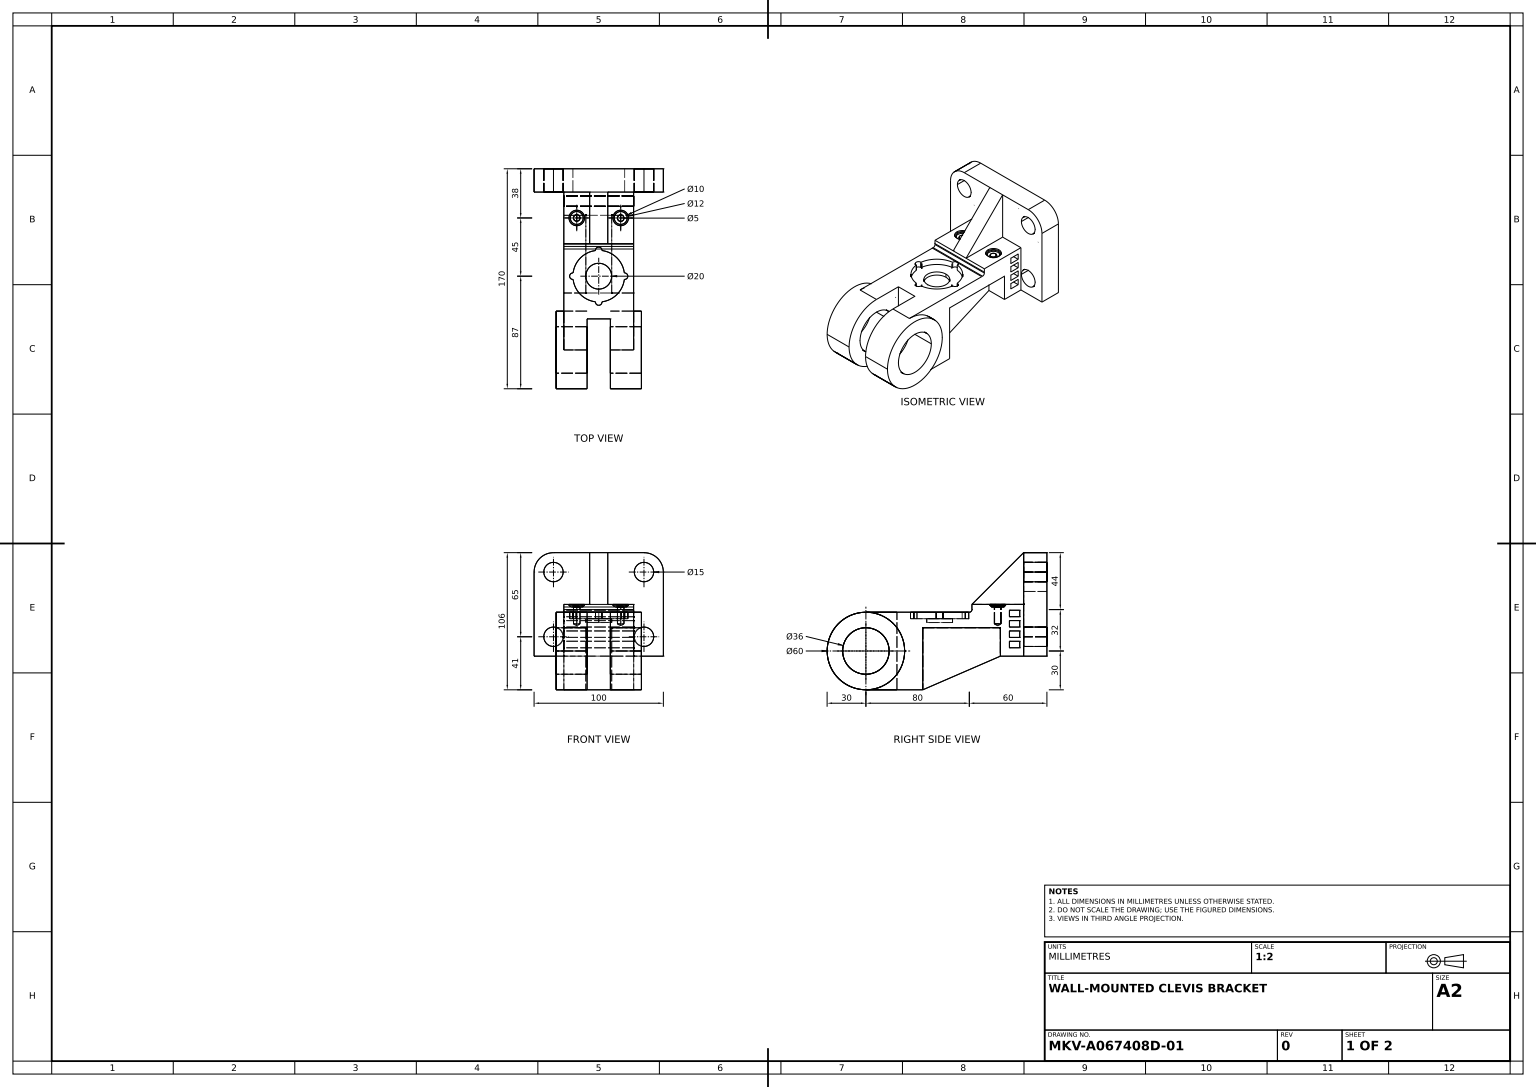
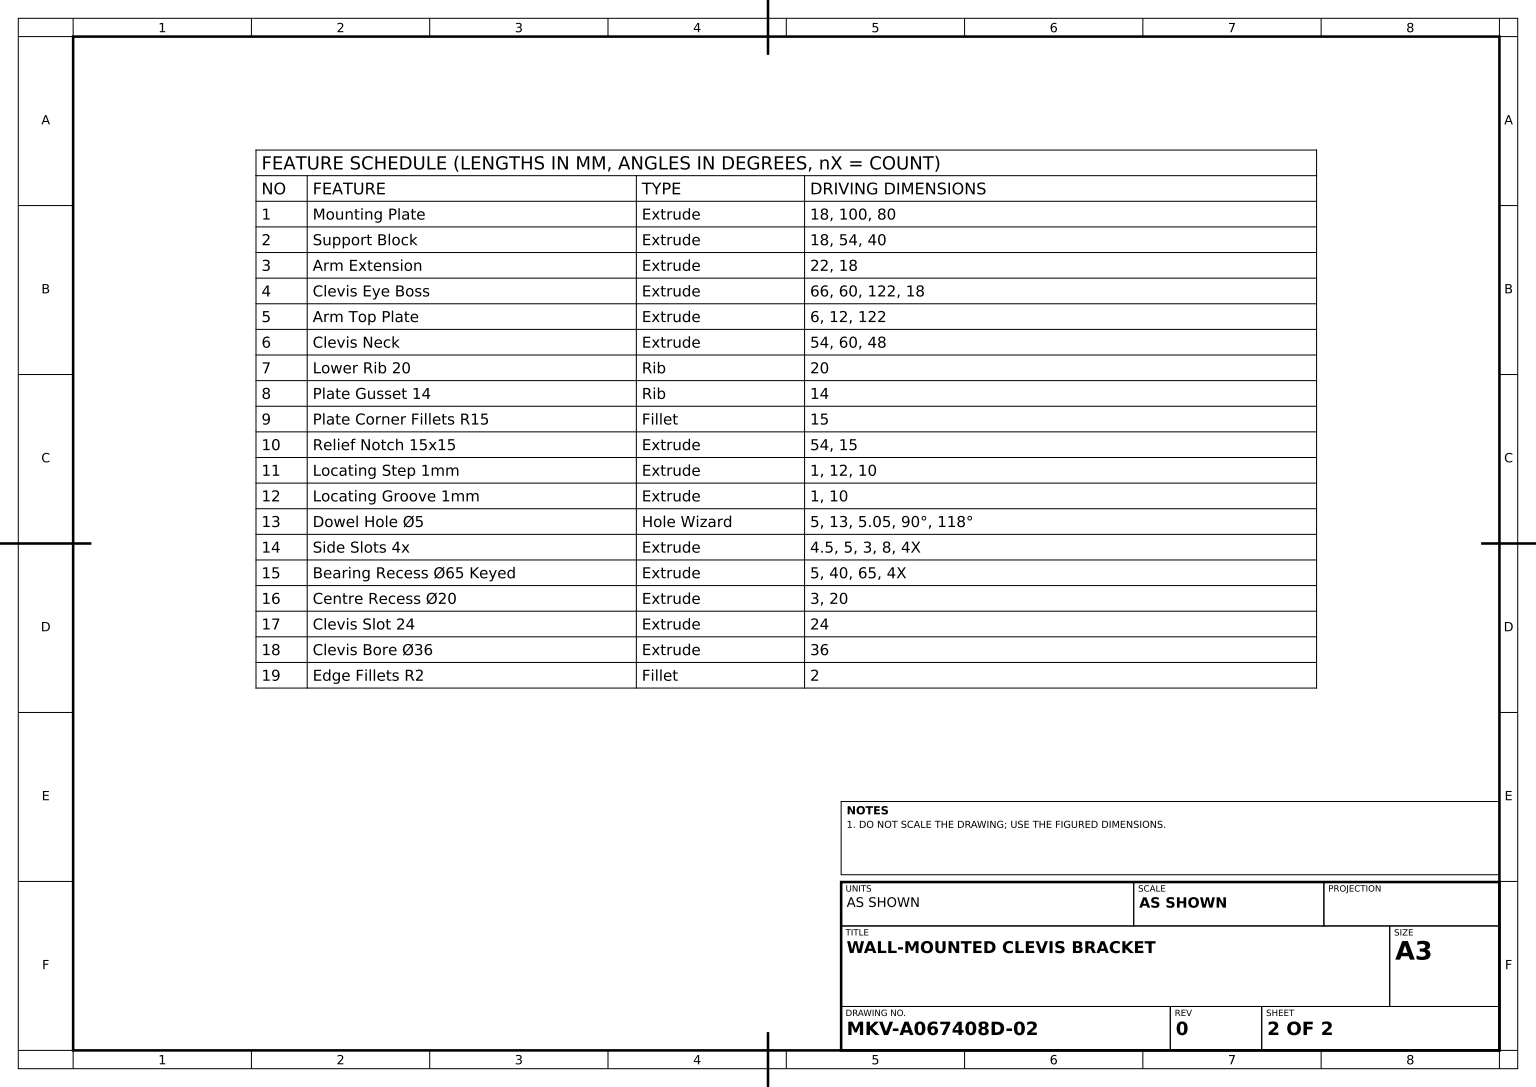
from build123d import *

# Parameters (mm, degrees)
MOUNTING_PLATE_SKETCH_W       = 100
MOUNTING_PLATE_SKETCH_H       = 80
MOUNTING_PLATE_DEPTH          = 18
SUPPORT_BLOCK_SKETCH_W        = 54
SUPPORT_BLOCK_SKETCH_H        = 40
SUPPORT_BLOCK_DEPTH           = 18
ARM_EXTENSION_SKETCH_W        = 54
ARM_EXTENSION_SKETCH_H        = 18
ARM_EXTENSION_DEPTH           = 22
CLEVIS_EYE_SKETCH_R           = 30
CLEVIS_EYE_BOSS_DEPTH         = 33
ARM_TOP_PLATE_SKETCH_W        = 54
ARM_TOP_PLATE_SKETCH_H        = 82
ARM_TOP_PLATE_DEPTH           = 12
CLEVIS_NECK_SKETCH_W          = 44
CLEVIS_NECK_SKETCH_H          = 48
CLEVIS_NECK_DEPTH             = 54
LOWER_RIB_20_REACH            = 191.093
LOWER_RIB_SKETCH_WALL_W       = 445.576270742
LOWER_RIB_SKETCH_WALL_H       = 20
PLATE_GUSSET_14_REACH         = 191.093
PLATE_GUSSET_SKETCH_WALL_W    = 436.75368234
PLATE_GUSSET_SKETCH_WALL_H    = 14
PLATE_CORNER_FILLETS_R15_R    = 15
RELIEF_NOTCH_SKETCH_R         = 7.5
RELIEF_NOTCH_15X15_DEPTH      = 54
LOCATING_STEP_SKETCH_R        = 6
LOCATING_STEP_1MM_DEPTH       = 1
LOCATING_GROOVE_SKETCH_R      = 5
LOCATING_GROOVE_1MM_DEPTH     = 1
DOWEL_HOLE_5_D                = 5
DOWEL_HOLE_5_DEPTH            = 13
DOWEL_HOLE_5_CSINK_D          = 5.05
DOWEL_HOLE_5_CSINK_ANGLE      = 90
DOWEL_HOLE_5_TIP              = 1.502151548
SIDE_SLOTS_SKETCH_W           = 8
SIDE_SLOTS_SKETCH_H           = 5
SIDE_SLOTS_4X_DEPTH           = 198.952014387
BEARING_RECESS_65_KEYED_DEPTH = 5
CENTRE_RECESS_SKETCH_R        = 10
CENTRE_RECESS_20_DEPTH        = 3
CLEVIS_SLOT_SKETCH_W          = 18
CLEVIS_SLOT_SKETCH_H          = 73.376983309
CLEVIS_SLOT_24_DEPTH          = 188.082869339
CLEVIS_BORE_SKETCH_R          = 18
CLEVIS_BORE_36_DEPTH          = 201.362172078
EDGE_FILLETS_R2_R             = 2


with BuildPart() as part:
    # Mounting Plate Sketch → Mounting Plate (new body)
    with BuildSketch(Plane.XY):
        Rectangle(MOUNTING_PLATE_SKETCH_W, MOUNTING_PLATE_SKETCH_H)
    extrude(amount=MOUNTING_PLATE_DEPTH)

    # Support Block Sketch → Support Block (add)
    with BuildSketch(Plane.XY.offset(18)):
        with Locations((0, -20)):
            Rectangle(SUPPORT_BLOCK_SKETCH_W, SUPPORT_BLOCK_SKETCH_H)
    extrude(amount=SUPPORT_BLOCK_DEPTH)

    # Arm Extension Sketch → Arm Extension (add)
    with BuildSketch(Plane.XY.offset(36)):
        with Locations((0, -9)):
            Rectangle(ARM_EXTENSION_SKETCH_W, ARM_EXTENSION_SKETCH_H)
    extrude(amount=ARM_EXTENSION_DEPTH)



with BuildPart() as body_2:
    # Clevis Eye Sketch → Clevis Eye Boss (new, symmetric)
    with BuildSketch(Plane(origin=(0, 0, 0), x_dir=(0, 0, -1), z_dir=(1, 0, 0))):
        with Locations((-140, -36)):
            Circle(CLEVIS_EYE_SKETCH_R)
    extrude(amount=CLEVIS_EYE_BOSS_DEPTH, both=True)


with BuildPart() as part_1:
    add(part.part)

    add(body_2.part)  # Arm Top Plate merges body 2
    # Arm Top Plate Sketch → Arm Top Plate (add)
    with BuildSketch(Plane(origin=(0, -6, 0), x_dir=(1, 0, 0), z_dir=(0, 1, 0))):
        with Locations((0, -99)):
            Rectangle(ARM_TOP_PLATE_SKETCH_W, ARM_TOP_PLATE_SKETCH_H)
    extrude(amount=-ARM_TOP_PLATE_DEPTH)

    # Clevis Neck Sketch → Clevis Neck (add)
    with BuildSketch(Plane.ZY.offset(27)):
        with Locations((118, -42)):
            Rectangle(CLEVIS_NECK_SKETCH_W, CLEVIS_NECK_SKETCH_H)
    extrude(amount=-CLEVIS_NECK_DEPTH)

    # Lower Rib Sketch wall → Lower Rib 20 (add, up to next)
    with BuildSketch(Plane(origin=(0, -53, 66), x_dir=(0, -0.397607437634, 0.91755562531), z_dir=(0, -0.91755562531, -0.397607437634)), mode=Mode.PRIVATE) as lower_rib_20_sk1:
        Rectangle(LOWER_RIB_SKETCH_WALL_W, LOWER_RIB_SKETCH_WALL_H)
    lower_rib_20_tool1 = extrude(lower_rib_20_sk1.sketch, amount=-LOWER_RIB_20_REACH, mode=Mode.PRIVATE) - part_1.part
    add(lower_rib_20_tool1.solids().sort_by_distance((0, -53, 66))[0])

    # Plate Gusset Sketch wall → Plate Gusset 14 (add, up to next)
    with BuildSketch(Plane(origin=(0, 20, 38), x_dir=(0, -0.707106781187, 0.707106781187), z_dir=(0, -0.707106781187, -0.707106781187)), mode=Mode.PRIVATE) as plate_gusset_14_sk1:
        Rectangle(PLATE_GUSSET_SKETCH_WALL_W, PLATE_GUSSET_SKETCH_WALL_H)
    plate_gusset_14_tool1 = extrude(plate_gusset_14_sk1.sketch, amount=PLATE_GUSSET_14_REACH, mode=Mode.PRIVATE) - part_1.part
    add(plate_gusset_14_tool1.solids().sort_by_distance((0, 20, 38))[0])

    # Plate Corner Fillets R15
    plate_corner_fillets_r15_edges = [part_1.edges().sort_by_distance(p)[0] for p in [
        (-50, 40, 9),
        (50, 40, 9),
    ]]
    fillet(plate_corner_fillets_r15_edges, radius=PLATE_CORNER_FILLETS_R15_R)

    # Relief Notch Sketch → Relief Notch 15x15 (cut)
    with BuildSketch(Plane.XY.offset(18)):
        with Locations((-35, 25)):
            Circle(RELIEF_NOTCH_SKETCH_R)
        with Locations((-35, -25)):
            Circle(RELIEF_NOTCH_SKETCH_R)
        with Locations((35, 25)):
            Circle(RELIEF_NOTCH_SKETCH_R)
        with Locations((35, -25)):
            Circle(RELIEF_NOTCH_SKETCH_R)
    extrude(amount=-RELIEF_NOTCH_15X15_DEPTH, mode=Mode.SUBTRACT)

    # Locating Step Sketch → Locating Step 1mm (cut)
    with BuildSketch(Plane(origin=(0, 0, 0), x_dir=(1, 0, 0), z_dir=(0, 1, 0))):
        with Locations(Location((-17, -38, 0), (0, 0, 180))):
            Circle(LOCATING_STEP_SKETCH_R)
        with Locations(Location((17, -38, 0), (0, 0, 180))):
            Circle(LOCATING_STEP_SKETCH_R)
    extrude(amount=-LOCATING_STEP_1MM_DEPTH, mode=Mode.SUBTRACT)

    # Locating Groove Sketch → Locating Groove 1mm (cut)
    with BuildSketch(Plane(origin=(0, -1, 0), x_dir=(1, 0, 0), z_dir=(0, 1, 0))):
        with Locations(Location((-17, -38, 0), (0, 0, 180))):
            Circle(LOCATING_GROOVE_SKETCH_R)
        with Locations(Location((17, -38, 0), (0, 0, 180))):
            Circle(LOCATING_GROOVE_SKETCH_R)
    extrude(amount=-LOCATING_GROOVE_1MM_DEPTH, mode=Mode.SUBTRACT)

    # Dowel Hole Ø5
    with Locations(Plane(origin=(0, -2, 0), x_dir=(1, 0, 0), z_dir=(0, 1, 0))):
        with Locations((-17, -38), (17, -38.121872411)):
            CounterSinkHole(DOWEL_HOLE_5_D / 2, DOWEL_HOLE_5_CSINK_D / 2, depth=DOWEL_HOLE_5_DEPTH, counter_sink_angle=DOWEL_HOLE_5_CSINK_ANGLE)
            with Locations((0, 0, -(DOWEL_HOLE_5_DEPTH + DOWEL_HOLE_5_TIP / 2))):  # 118° drill point
                Cone(0, DOWEL_HOLE_5_D / 2, DOWEL_HOLE_5_TIP, mode=Mode.SUBTRACT)

    # Side Slots Sketch → Side Slots 4x (cut, through all)
    with BuildSketch(Plane.ZY.offset(27)):
        with Locations((25, -7)):
            Rectangle(SIDE_SLOTS_SKETCH_W, SIDE_SLOTS_SKETCH_H)
        with Locations((25, -15)):
            Rectangle(SIDE_SLOTS_SKETCH_W, SIDE_SLOTS_SKETCH_H)
        with Locations((25, -23)):
            Rectangle(SIDE_SLOTS_SKETCH_W, SIDE_SLOTS_SKETCH_H)
        with Locations((25, -31)):
            Rectangle(SIDE_SLOTS_SKETCH_W, SIDE_SLOTS_SKETCH_H)
    extrude(amount=-SIDE_SLOTS_4X_DEPTH, mode=Mode.SUBTRACT)

    # Bearing Recess Sketch → Bearing Recess Ø65 Keyed (cut)
    with BuildSketch(Plane(origin=(0, -6, 0), x_dir=(1, 0, 0), z_dir=(0, 1, 0))):
        with BuildLine():
            ThreePointArc((-19.84375, -85.49511241), (-14.142135624, -97.142135624), (-2.49511241, -102.84375))
            ThreePointArc((-2.49511241, -102.84375), (0, -105.5), (2.49511241, -102.84375))
            ThreePointArc((2.49511241, -102.84375), (14.142135624, -97.142135624), (19.84375, -85.49511241))
            ThreePointArc((19.84375, -85.49511241), (22.5, -83), (19.84375, -80.50488759))
            ThreePointArc((19.84375, -80.50488759), (14.142135624, -68.857864376), (2.49511241, -63.15625))
            ThreePointArc((2.49511241, -63.15625), (0, -60.5), (-2.49511241, -63.15625))
            ThreePointArc((-2.49511241, -63.15625), (-14.142135624, -68.857864376), (-19.84375, -80.50488759))
            ThreePointArc((-19.84375, -80.50488759), (-22.5, -83), (-19.84375, -85.49511241))
        make_face()
    extrude(amount=-BEARING_RECESS_65_KEYED_DEPTH, mode=Mode.SUBTRACT)

    # Centre Recess Sketch → Centre Recess Ø20 (cut)
    with BuildSketch(Plane(origin=(0, -11, 0), x_dir=(1, 0, 0), z_dir=(0, 1, 0))):
        with Locations(Location((0, -83, 0), (0, 0, 270))):
            Circle(CENTRE_RECESS_SKETCH_R)
    extrude(amount=-CENTRE_RECESS_20_DEPTH, mode=Mode.SUBTRACT)

    # Clevis Slot Sketch → Clevis Slot 24 (cut, through all)
    with BuildSketch(Plane(origin=(0, -6, 0), x_dir=(1, 0, 0), z_dir=(0, 1, 0))):
        with Locations((0, -152.688491655)):
            Rectangle(CLEVIS_SLOT_SKETCH_W, CLEVIS_SLOT_SKETCH_H)
    extrude(amount=-CLEVIS_SLOT_24_DEPTH, mode=Mode.SUBTRACT)

    # Clevis Bore Sketch → Clevis Bore Ø36 (cut, through all)
    with BuildSketch(Plane.ZY.offset(33)):
        with Locations(Location((140, -36, 0), (0, 0, 180))):
            Circle(CLEVIS_BORE_SKETCH_R)
    extrude(amount=-CLEVIS_BORE_36_DEPTH, mode=Mode.SUBTRACT)

    # Edge Fillets R2
    edge_fillets_r2_edges = [part_1.edges().sort_by_distance(p)[0] for p in [
        (0, -6, 58),
    ]]
    fillet(edge_fillets_r2_edges, radius=EDGE_FILLETS_R2_R)


solid = part_1.part
